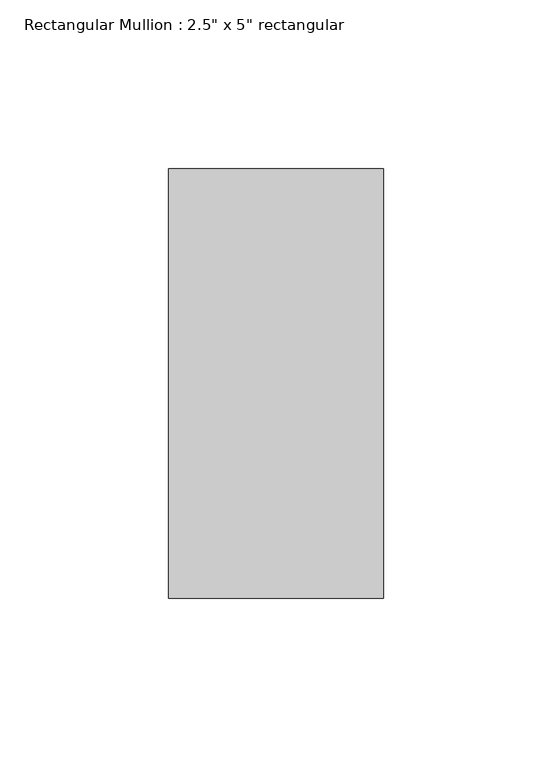
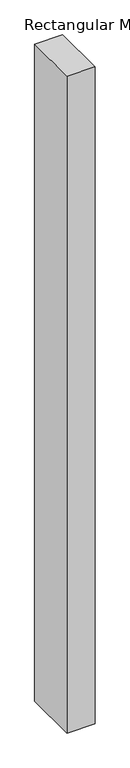
"""IFC4 building model written with IfcOpenShell, lengths in millimetres: member geometry."""

from ifc_helpers import new_model, si_unit, frame, origin, place, context, project, spatial, polyline, outline, extrude, source, transform, mapped, element, save


def member_65d07e0b(model_context):
    return source(origin(), model_context, "Body", "SweptSolid", [
        extrude(outline(polyline([(0.0, 63.5), (0.0, -63.5), (-63.5, -63.5), (-63.5, 63.5), (0.0, 63.5)])), frame((0.0, 0.0, -1576.8375758), z_axis=(0.0, 0.0, 1.0), x_axis=(1.0, 0.0, 0.0)), (0.0, 0.0, 1.0), 1576.8375758),
    ])


if __name__ == "__main__":
    model = new_model("IFC4")
    model_context = context("Model", 3, world=origin())
    ifc_project = project(units=[si_unit("LENGTHUNIT", "METRE", prefix="MILLI")], contexts=[model_context])
    site = spatial("IfcSite", under=ifc_project)
    building = spatial("IfcBuilding", under=site)
    placement = place(None, origin())
    member_shape = member_65d07e0b(model_context)
    element("IfcMember", 1, ObjectType="Rectangular Mullion : 2.5\" x 5\" rectangular", at=placement, inside=building, context=model_context, shape_type="MappedRepresentation", body=[
        mapped(member_shape, transform((0.0, 0.0, 0.0), x_axis=(1.0, 0.0, 0.0), y_axis=(0.0, 1.0, 0.0), z_axis=(0.0, 0.0, 1.0))),
    ])
    save(model, "model.ifc")

# Revit data of these elements
# Type "Rectangular Mullion : 2.5\" x 5\" rectangular"
#   built-in parameter 1007304 = 0.416667 (stored number, unit not read)
#   built-in parameter 1007301 = 0.104167 (stored number, unit not read)
#   built-in parameter 1007300 = 0.104167 (stored number, unit not read)
# Element 1 (IfcMember, "Rectangular Mullion : 2.5\" x 5\" rectangular")
#   Materials on its faces: "Aluminum"
# Materials
#   "Aluminum": class "Metal", colour RGB 247 247 247, transparency 0, Description = "Aluminum 6061", Cost = 0
